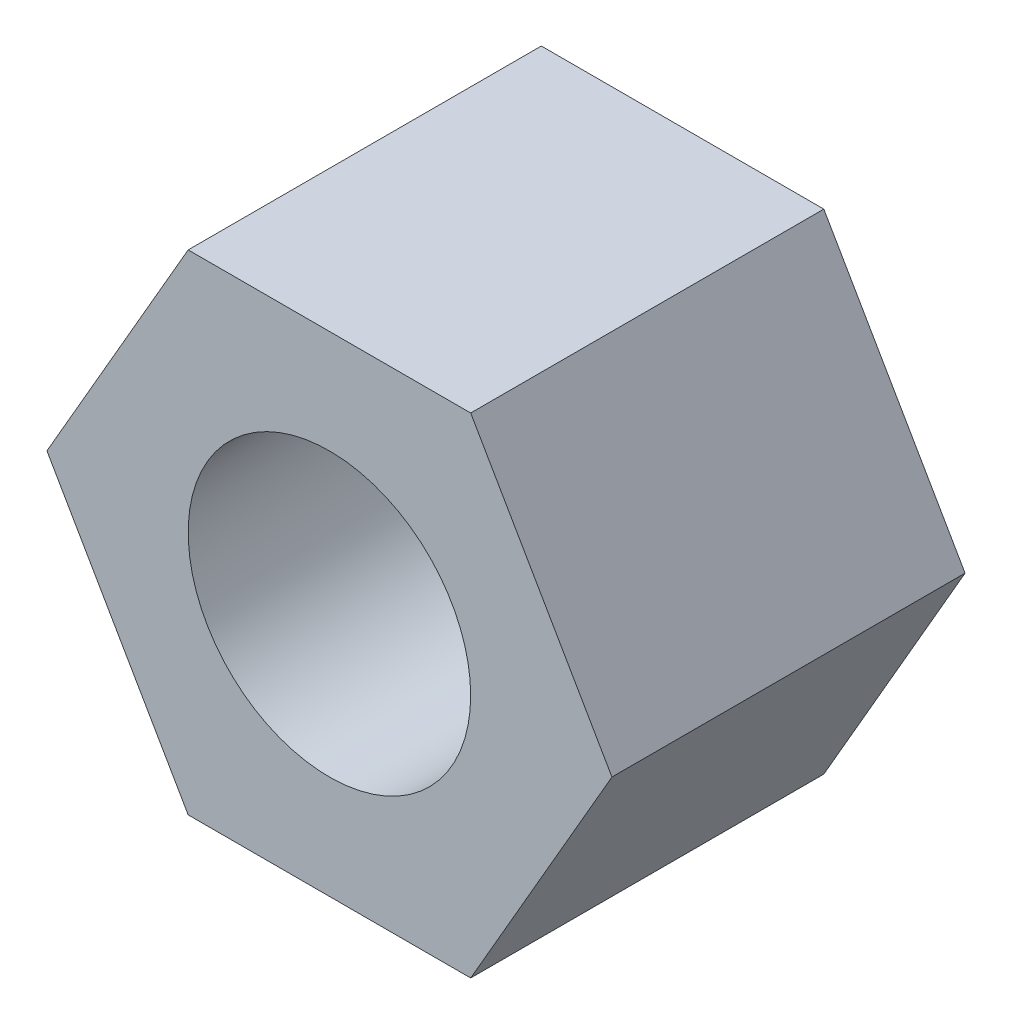
from build123d import *

# Parameters (mm, degrees)
HEX_PROFILE_WITH_BORE_12_R = 6
HEX_BODY_15MM_DEPTH        = 15


with BuildPart() as part:
    # Hex Profile with Bore Ø12 → Hex Body 15mm (new body)
    with BuildSketch(Plane.XY):
        Polygon((12, 0), (6, 10.392304845), (-6, 10.392304845), (-12, 0), (-6, -10.392304845), (6, -10.392304845), align=None)
        Circle(HEX_PROFILE_WITH_BORE_12_R, mode=Mode.SUBTRACT)
    extrude(amount=HEX_BODY_15MM_DEPTH)


solid = part.part
